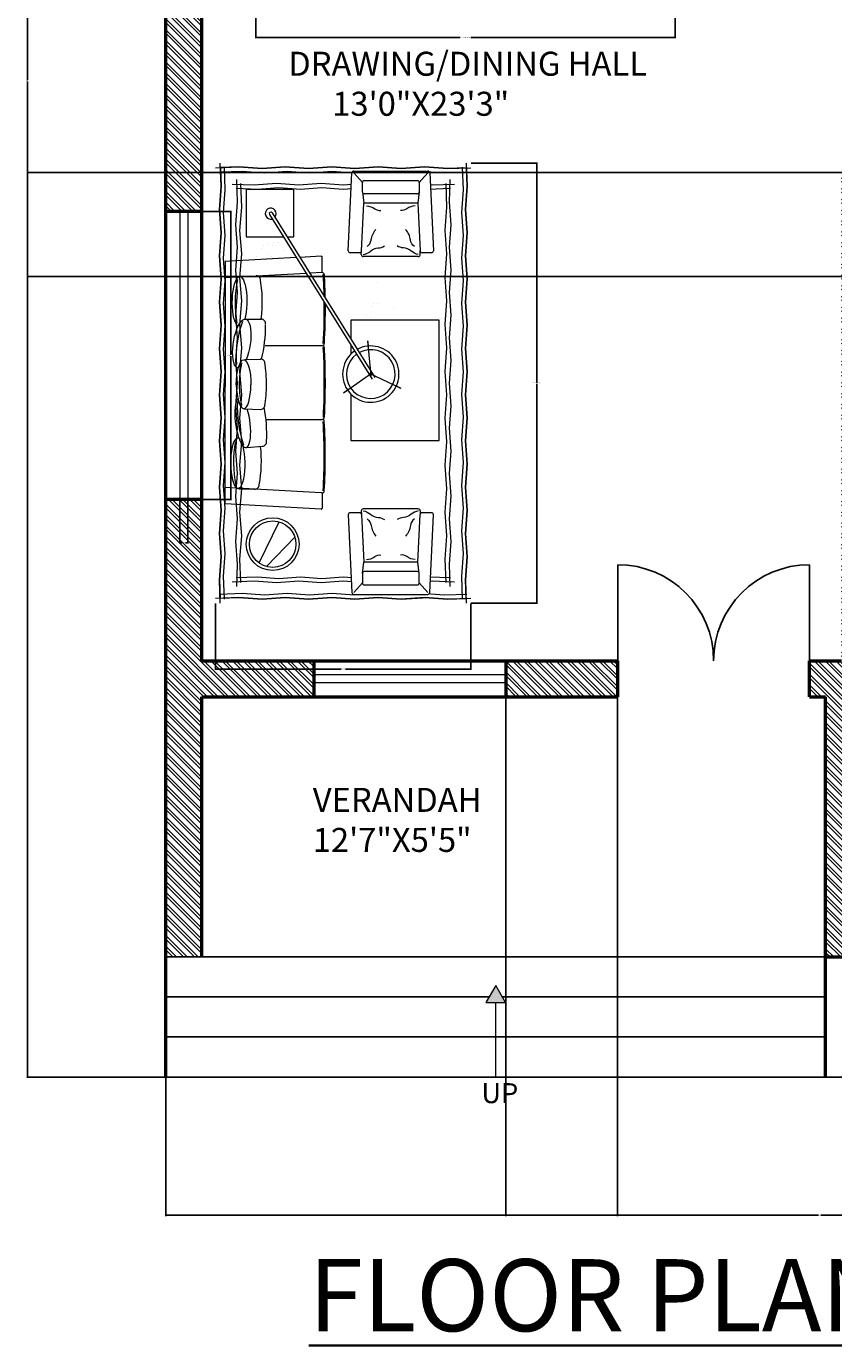
# Model space of a CAD drawing. Units: inches. Extents: x 10696 to 11614, y 5787 to 6498.
# Tile 1 of 9: x 10696 to 10898, y 5790 to 6120. Entities that reach past the tile are written whole.
import ezdxf

# ---------------------------------------------------------------- set-up
doc = ezdxf.new("R2010")
doc.units = ezdxf.units.IN
doc.set_wipeout_variables(frame=1)
for name, color, linetype, lineweight in [('A-ANNO-DIMS', 2, 'Continuous', 18), ('A-ANNO-SYMB', 2, 'Continuous', 18), ('A-ANNO-TITL', 7, 'Continuous', 35), ('A-AREA-IDEN', 7, 'Continuous', 25), ('A-DOOR', 3, 'Continuous', 25), ('A-FLOR', 7, 'Continuous', 25), ('A-FLOR-STRS', 7, 'Continuous', 25), ('A-FURN', 8, 'Continuous', 18), ('A-GLAZ', 4, 'Continuous', 20), ('A-WALL', 7, 'Continuous', 50), ('A-WALL-PATT', 252, 'Continuous', 13)]:
    doc.layers.add(name, color=color, linetype=linetype, lineweight=lineweight)
doc.styles.get("Standard").update_dxf_attribs({"font": 'arial.ttf'})
doc.dimstyles.get("Standard").update_dxf_attribs({"dimtxt": 0.18, "dimasz": 0.18, "dimexe": 0.18, "dimexo": 0.0625, "dimgap": 0.09, "dimtad": 0, "dimtih": 1, "dimtoh": 1, "dimdec": 4, "dimzin": 0, "dimdsep": 46, "dimtxsty": 'Standard', "dimcen": 0.09, "dimadec": 0, "dimazin": 0, "dimtfac": 1, "dimtdec": 4, "dimtofl": 0, "dimtmove": 0, "dimatfit": 3, "dimfxl": 1, "dimtolj": 1, "dimtzin": 0, "dimarcsym": 0})

# ---------------------------------------------------------------- blocks, each defined once
blk = doc.blocks.new('A$C7590614E')
for p, q in [((220, 4135), (46, 4129)), ((46, 4129), (52, 3952)), ((46, 4129), (46, 4129)), ((440, 4119), (220, 4135)), ((660, 4135), (440, 4119)), ((881, 4119), (660, 4135)), ((1101, 4135), (881, 4119)), ((1321, 4119), (1101, 4135)), ((1541, 4135), (1321, 4119)), ((1761, 4119), (1541, 4135)), ((1981, 4135), (1761, 4119)), ((2202, 4119), (1981, 4135)), ((2379, 4126), (2202, 4119)), ((2385, 3952), (2379, 4126)), ((52, 3952), (36, 3732)), ((2369, 3732), (2385, 3952)), ((36, 3732), (52, 3513)), ((2385, 3513), (2369, 3732)), ((52, 3513), (36, 3293)), ((496, 3597), (496, 3597)), ((596, 3620), (596, 3620)), ((2369, 3293), (2385, 3513)), ((454, 3393), (454, 3393)), ((492, 3396), (492, 3396)), ((536, 3390), (536, 3390)), ((553, 3416), (553, 3416)), ((592, 3420), (592, 3420)), ((36, 3293), (52, 3074)), ((765, 3275), (91, 3238)), ((392, 3284), (392, 3284)), ((426, 3262), (426, 3262)), ((436, 3366), (436, 3366)), ((492, 3308), (492, 3308)), ((526, 3286), (526, 3286)), ((641, 3347), (641, 3347)), ((741, 3371), (741, 3371)), ((1000, 3288), (799, 3277)), ((1011, 3134), (1011, 3278)), ((2385, 3074), (2369, 3293)), ((91, 3238), (91, 2051)), ((91, 3161), (91, 2051)), ((1010, 3133), (893, 3127)), ((52, 3074), (37, 2858)), ((859, 3125), (91, 3084)), ((236, 3098), (385, 3104)), ((374, 3100), (240, 3093)), ((332, 3098), (253, 3094)), ((1538, 3041), (1538, 3041)), ((2369, 2854), (2385, 3074)), ((37, 2858), (52, 2635)), ((1479, 2810), (1479, 2810)), ((1496, 2837), (1496, 2837)), ((1535, 2840), (1535, 2840)), ((1683, 2791), (1683, 2791)), ((2385, 2635), (2369, 2854)), ((52, 2635), (36, 2415)), ((276, 2693), (435, 2692)), ((1434, 2729), (1434, 2729)), ((1469, 2706), (1469, 2706)), ((2369, 2415), (2385, 2635)), ((36, 2415), (52, 2196)), ((469, 2441), (1012, 2441)), ((2385, 2196), (2369, 2415)), ((275, 2308), (424, 2314)), ((52, 2196), (36, 1976)), ((2369, 1976), (2385, 2196)), ((91, 941), (91, 2051)), ((91, 941), (91, 2051)), ((36, 1976), (52, 1756)), ((2385, 1756), (2369, 1976)), ((52, 1756), (36, 1537)), ((275, 1842), (424, 1836)), ((2369, 1537), (2385, 1756)), ((478, 1742), (1012, 1742)), ((36, 1537), (52, 1317)), ((2385, 1317), (2369, 1537)), ((296, 1474), (445, 1487)), ((52, 1317), (36, 1098)), ((2369, 1098), (2385, 1317)), ((36, 1098), (52, 878)), ((1001, 1045), (91, 1095)), ((221, 1085), (370, 1080)), ((1010, 1045), (1001, 1045)), ((1011, 1045), (1011, 901)), ((2385, 878), (2369, 1098)), ((52, 878), (36, 659)), ((1001, 891), (91, 941)), ((2369, 659), (2385, 878)), ((36, 659), (52, 439)), ((2385, 439), (2369, 659)), ((52, 439), (36, 220)), ((2369, 220), (2385, 439)), ((36, 220), (43, 46)), ((2376, 43), (2369, 220)), ((43, 46), (220, 52)), ((220, 52), (440, 36)), ((440, 36), (660, 52)), ((660, 52), (881, 36)), ((881, 36), (1101, 52)), ((1101, 52), (1321, 36)), ((1321, 36), (1541, 52)), ((1541, 52), (1761, 36)), ((1761, 36), (1966, 51)), ((1966, 51), (1981, 52)), ((1981, 52), (2202, 36)), ((2202, 36), (2376, 43))]:
    blk.add_line(p, q)
at = {"linetype": 'ByBlock'}
for p, q in [((1474, 2154, 0), (1445, 2485, 0)), ((1474, 2154, 0), (1445, 2485, 0)), ((1450, 2427, 0), (1446, 2481, 0)), ((1487, 2182, 0), (1213, 1991, 0)), ((1487, 2182, 0), (1213, 1991, 0)), ((1456, 2179, 0), (1757, 2037, 0)), ((1456, 2179, 0), (1757, 2037, 0)), ((1261, 2025, 0), (1217, 1994, 0)), ((1705, 2062, 0), (1754, 2039, 0)), ((412, 381), (604, 770)), ((751, 626), (481, 348))]:
    blk.add_line(p, q, dxfattribs=at)
at = {"linetype": 'ByBlock', "flags": 128}
for points in [[(0, 4127), (220, 4135), (440, 4119), (660, 4135), (881, 4119), (1101, 4135), (1321, 4119), (1541, 4135), (1761, 4119), (1981, 4135), (2202, 4119), (2422, 4127)], [(44, 0), (36, 220), (52, 439), (36, 659), (52, 878), (36, 1098), (52, 1317), (36, 1537), (52, 1756), (36, 1976), (52, 2196), (36, 2415), (52, 2635), (36, 2854), (52, 3074), (36, 3293), (52, 3513), (36, 3732), (52, 3952), (44, 4172)], [(83, 39), (75, 254), (91, 470), (75, 685), (91, 901), (75, 1116), (91, 1332), (75, 1547), (91, 1763), (75, 1978), (91, 2194), (75, 2409), (91, 2624), (75, 2840), (91, 3055), (75, 3271), (91, 3486), (75, 3702), (91, 3917), (83, 4133)], [(2339, 4133), (2347, 3917), (2331, 3702), (2347, 3486), (2331, 3271), (2347, 3055), (2331, 2840), (2347, 2624), (2331, 2409), (2347, 2194), (2331, 1978), (2347, 1763), (2331, 1547), (2347, 1332), (2331, 1116), (2347, 901), (2331, 685), (2347, 470), (2331, 254), (2339, 39)], [(2377, 4172), (2385, 3952), (2369, 3732), (2385, 3513), (2369, 3293), (2385, 3074), (2369, 2854), (2385, 2635), (2369, 2415), (2385, 2196), (2369, 1976), (2385, 1756), (2369, 1537), (2385, 1317), (2369, 1098), (2385, 878), (2369, 659), (2385, 439), (2369, 220), (2377, 0)], [(39, 4088), (252, 4096), (465, 4080), (678, 4096), (891, 4080), (1104, 4096), (1317, 4080), (1531, 4096), (1744, 4080), (1957, 4096), (2170, 4080), (2383, 4088)], [(200, 156), (208, 370), (192, 584), (208, 799), (192, 1013), (208, 1228), (192, 1442), (208, 1657), (192, 1871), (208, 2086), (192, 2300), (208, 2515), (192, 2729), (208, 2944), (192, 3158), (208, 3373), (192, 3587), (208, 3802), (200, 4016)], [(2222, 4016), (2214, 3802), (2230, 3587), (2214, 3373), (2230, 3158), (2214, 2944), (2230, 2729), (2214, 2515), (2230, 2300), (2214, 2086), (2230, 1871), (2214, 1657), (2230, 1442), (2214, 1228), (2230, 1013), (2214, 799), (2230, 584), (2214, 370), (2222, 156)], [(156, 3972), (367, 3964), (578, 3980), (789, 3964), (1000, 3980), (1211, 3964), (1422, 3980), (1633, 3964), (1844, 3980), (2055, 3964), (2266, 3972)], [(194, 3933), (398, 3925), (601, 3941), (804, 3925), (1008, 3941), (1211, 3925), (1414, 3941), (1617, 3925), (1821, 3941), (2024, 3925), (2227, 3933)], [(239, 194), (231, 417), (247, 639), (231, 862), (247, 1084), (231, 1307), (247, 1529), (231, 1752), (247, 1975), (231, 2197), (247, 2420), (231, 2642), (247, 2865), (231, 3087), (247, 3310), (231, 3532), (247, 3755), (239, 3977)], [(2183, 3977), (2191, 3755), (2175, 3532), (2191, 3310), (2175, 3087), (2191, 2865), (2175, 2642), (2191, 2420), (2175, 2197), (2191, 1975), (2175, 1752), (2191, 1529), (2175, 1307), (2191, 1084), (2175, 862), (2191, 639), (2175, 417), (2183, 194)], [(2266, 200), (2055, 208), (1844, 192), (1633, 208), (1422, 192), (1211, 208), (1000, 192), (789, 208), (578, 192), (367, 208), (156, 200)], [(2227, 239), (2024, 247), (1821, 231), (1617, 247), (1414, 231), (1211, 247), (1008, 231), (804, 247), (601, 231), (398, 247), (194, 239)], [(2422, 44), (2202, 36), (1981, 52), (1761, 36), (1541, 52), (1321, 36), (1101, 52), (881, 36), (660, 52), (440, 36), (220, 52), (0, 44)], [(2383, 83), (2170, 75), (1957, 91), (1744, 75), (1531, 91), (1317, 75), (1104, 91), (891, 75), (678, 91), (465, 75), (252, 91), (39, 83)]]:
    blk.add_lwpolyline(points, dxfattribs=at)
at = {"linetype": 'ByBlock'}
blk.add_lwpolyline([(678, 3471), (741, 3471), (741, 3921), (291, 3921), (291, 3471), (643, 3471)], dxfattribs=at)
for points in [[(1282, 1984), (1282, 1541), (2122, 1541), (2122, 2681), (1282, 2681), (1282, 2504)], [(1282, 2447), (1282, 2359)]]:
    blk.add_lwpolyline(points)
at = {"linetype": 'ByBlock', "const_width": 10, "elevation": 0}
for points in [[(1450, 2427), (1446, 2481)], [(1261, 2025), (1217, 1994)], [(1705, 2062), (1754, 2039)]]:
    blk.add_lwpolyline(points, dxfattribs=at)
at = {"linetype": 'ByBlock'}
for radius in [250, 220]:
    blk.add_circle((541, 559), radius, dxfattribs=at)
for radius, start, end in [(52.4, 318.5939, 285.3184), (15, 31.9562, 211.9562)]:
    blk.add_arc((523, 3692), radius, start, end, dxfattribs=at)
for centre, radius, start, end in [((1001, 3278), 10, 0, 93.0128), ((1011, 3113), 20, 3.7459, 93.0128), ((1254, 2846), 1070, 168.034, 190.3551), ((-385, 2845), 798, 18.6145, 18.6419), ((387, 3061), 42.5, 33.8407, 92.0223), ((-822, 2855), 1265, 352.6106, 10.4711), ((-4595, 2788), 5626, 1.223, 3.3226), ((-4595, 2788), 5636, 1.0525, 3.3226), ((-4595, 2788), 5626, 356.669, 0.6303), ((-4595, 2788), 5636, 356.669, 0.4637), ((1265, 2321), 1070, 160.9121, 183.2331), ((431, 2650), 42.5, 352.6116, 84.9003), ((-796, 2619), 1269, 346.0345, 0.8134), ((1011, 2421), 20, 3.742, 91.3972), ((1011, 2461), 20, 271.3972, 356.2445), ((-2252, 2185), 3282, 359.485, 4.1508), ((-2252, 2185), 3292, 359.485, 4.1508), ((1293, 2055), 1070, 168.034, 179.2769), ((425, 2271), 42.5, 16.3929, 92.0223), ((-783, 2085), 1265, 359.2714, 9.0059), ((425, 2271), 42.5, 359.7336, 1.1068), ((-4089, 2069), 5120, 356.563, 0.9635), ((-4089, 2069), 5130, 356.563, 0.9635), ((1293, 2094), 1070, 181.3636, 191.966), ((-783, 2065), 1265, 350.9941, 0.1868), ((1275, 1851), 1070, 176.7669, 199.0879), ((425, 1879), 42.5, 358.8932, 0.2664), ((425, 1879), 42.5, 267.9777, 343.6071), ((-780, 1606), 1265, 356.7804, 11.4363), ((1011, 1762), 20, 268.6028, 356.258), ((1011, 1722), 20, 3.7555, 88.6028), ((-4697, 1393), 5727, 356.706, 3.3024), ((-4697, 1393), 5737, 356.706, 3.3024), ((1239, 1338), 1070, 169.6449, 191.966), ((441, 1530), 42.5, 275.0997, 7.3884), ((-831, 1350), 1265, 349.6584, 6.1656), ((-400, 1339), 798, 341.3581, 341.3855), ((371, 1122), 42.5, 267.9777, 0.2664), ((1011, 1065), 20, 266.9872, 356.2541), ((1001, 901), 10, 266.9872, 0)]:
    blk.add_arc(centre, radius, start, end)
at = {"extrusion": (0, 0, -1)}
for centre, major_axis, ratio, start_param, end_param in [((227, 2858), (2, 239), 0.289653, 3.343252, 8.61472), ((248, 2460), (35, 232), 0.342983, 3.115548, 8.511087), ((265, 2068), (2, 239), 0.289653, -1.56819, 1.564113)]:
    blk.add_ellipse(centre, major_axis=major_axis, ratio=ratio, start_param=start_param, end_param=end_param, dxfattribs=at)
at = {"linetype": 'ByBlock', "extrusion": (3.38184e-09, 2.26187e-09, 1)}
for major_axis, start_param, end_param in [((-219, -153, 0), 4.720612, 10.891434), ((-190, -132, 0), 4.729628, 10.883141)]:
    blk.add_ellipse((1472, 2171), major_axis=major_axis, ratio=1, start_param=start_param, end_param=end_param, dxfattribs=at)
for centre, major_axis, start_param, end_param in [((265, 2082), (-2, 239), 1.623473, 4.655635), ((257, 1711), (-31, 237), 0.253375, 5.250818), ((211, 1326), (-2, 239), -0.16583, 5.452765)]:
    blk.add_ellipse(centre, major_axis=major_axis, ratio=0.289653, start_param=start_param, end_param=end_param)
for points in [[(1941, 3334), (1941, 3305), (1940, 3297), (1936, 3292), (1929, 3287), (1929, 3287), (1919, 3286), (1838, 3286), (1732, 3286), (1653, 3286), (1475, 3286), (1400, 3286), (1392, 3288), (1387, 3292), (1383, 3298), (1382, 3305), (1382, 3311), (1383, 3317), (1383, 3329), (1383, 3336), (1378, 3327), (1372, 3323), (1366, 3322), (1359, 3322), (1271, 3323), (1263, 3328), (1263, 3328), (1259, 3334), (1258, 3341), (1258, 3341), (1292, 4079), (1294, 4086), (1297, 4091), (1297, 4091), (1310, 4096), (1316, 4096), (1326, 4096), (1336, 4096), (2002, 4096), (2014, 4096), (2026, 4091), (2032, 4079), (2032, 4070), (2066, 3341), (2061, 3328), (2061, 3328), (2048, 3322), (2028, 3322), (1992, 3322), (1958, 3322), (1951, 3324), (1945, 3327), (1944, 3329)], [(1941, 845), (1941, 874), (1940, 882), (1936, 887), (1929, 892), (1929, 892), (1919, 893), (1838, 893), (1732, 893), (1653, 893), (1475, 893), (1400, 893), (1392, 891), (1387, 887), (1383, 881), (1382, 874), (1382, 868), (1383, 862), (1383, 850), (1383, 843), (1378, 852), (1372, 856), (1366, 857), (1359, 857), (1271, 856), (1263, 851), (1263, 851), (1259, 845), (1258, 838), (1258, 838), (1292, 100), (1294, 93), (1297, 88), (1297, 88), (1310, 83), (1316, 83), (1326, 83), (1336, 83), (2002, 83), (2014, 83), (2026, 88), (2032, 100), (2032, 109), (2066, 838), (2061, 851), (2061, 851), (2048, 857), (2028, 857), (1992, 857), (1958, 857), (1951, 855), (1945, 852), (1944, 850)]]:
    blk.add_wipeout(points).translate(0, 0, 0)
at = {"linetype": 'ByBlock'}
for p, q in [((1258, 3341, 0), (1292, 4079, 0)), ((1310, 4096, 0), (2014, 4096, 0)), ((1310, 4078, 0), (1392, 3988, 0)), ((1310, 4078, 0), (1392, 3988, 0)), ((1410, 4006, 0), (1914, 4006, 0)), ((1410, 4006, 0), (1914, 4006, 0)), ((2014, 4078, 0), (1932, 3988, 0)), ((2014, 4078, 0), (1932, 3988, 0)), ((2032, 4079, 0), (2066, 3341, 0)), ((1392, 3898, 0), (1392, 3988, 0)), ((1392, 3898, 0), (1392, 3988, 0)), ((1392, 3898, 0), (1405, 3792, 0)), ((1392, 3898, 0), (1405, 3792, 0)), ((1914, 3880, 0), (1410, 3880, 0)), ((1914, 3880, 0), (1410, 3880, 0)), ((1932, 3898, 0), (1919, 3792, 0)), ((1932, 3898, 0), (1919, 3792, 0)), ((1932, 3988, 0), (1932, 3898, 0)), ((1932, 3988, 0), (1932, 3898, 0)), ((1384, 3339, 0), (1405, 3792, 0)), ((1384, 3339, 0), (1405, 3792, 0)), ((1919, 3792, 0), (1405, 3792, 0)), ((1919, 3792, 0), (1405, 3792, 0)), ((1919, 3792, 0), (1940, 3339, 0)), ((1919, 3792, 0), (1940, 3339, 0)), ((510, 3684), (1484, 2123)), ((536, 3700), (1510, 2138)), ((1366, 3322, 0), (1276, 3322, 0)), ((1382, 3305, 0), (1384, 3339, 0)), ((1923, 3286, 0), (1400, 3286, 0)), ((1941, 3305, 0), (1940, 3339, 0)), ((2048, 3322, 0), (1958, 3322, 0)), ((1923, 893, 0), (1400, 893, 0)), ((1258, 838, 0), (1292, 100, 0)), ((1366, 857, 0), (1276, 857, 0)), ((1382, 874, 0), (1384, 840, 0)), ((1384, 840, 0), (1405, 387, 0)), ((1384, 840, 0), (1405, 387, 0)), ((1919, 387, 0), (1940, 840, 0)), ((1919, 387, 0), (1940, 840, 0)), ((1941, 874, 0), (1940, 840, 0)), ((2048, 857, 0), (1958, 857, 0)), ((2032, 100, 0), (2066, 838, 0)), ((1392, 281, 0), (1405, 387, 0)), ((1392, 281, 0), (1405, 387, 0)), ((1919, 387, 0), (1405, 387, 0)), ((1919, 387, 0), (1405, 387, 0)), ((1932, 281, 0), (1919, 387, 0)), ((1932, 281, 0), (1919, 387, 0)), ((1392, 281, 0), (1392, 191, 0)), ((1392, 281, 0), (1392, 191, 0)), ((1914, 299, 0), (1410, 299, 0)), ((1914, 299, 0), (1410, 299, 0)), ((1932, 191, 0), (1932, 281, 0)), ((1932, 191, 0), (1932, 281, 0)), ((1310, 101, 0), (1392, 191, 0)), ((1310, 101, 0), (1392, 191, 0)), ((1410, 173, 0), (1914, 173, 0)), ((1410, 173, 0), (1914, 173, 0)), ((2014, 101, 0), (1932, 191, 0)), ((2014, 101, 0), (1932, 191, 0)), ((1310, 83, 0), (2014, 83, 0))]:
    blk.add_line(p, q, dxfattribs=at)
at = {"linetype": 'ByBlock', "elevation": 0}
for points in [[(1430, 3765, -0.157856), (1510, 3738, 0.195258), (1568, 3723, 0.506042)], [(1430, 3765, -0.157856), (1510, 3738, 0.195258), (1568, 3723, 0.506042)], [(1894, 3765, 0.157856), (1813, 3738, -0.195258), (1755, 3723, -0.506042)], [(1894, 3765, 0.157856), (1813, 3738, -0.195258), (1755, 3723, -0.506042)], [(1437, 3380, 0.215808), (1475, 3442, -0.158378), (1521, 3543, -0.75133)], [(1437, 3380, 0.215808), (1475, 3442, -0.158378), (1521, 3543, -0.75133)], [(1886, 3380, -0.215808), (1849, 3442, 0.158378), (1802, 3543, 0.75133)], [(1886, 3380, -0.215808), (1849, 3442, 0.158378), (1802, 3543, 0.75133)], [(1400, 3304, 0.13045), (1468, 3337, -0.166434), (1542, 3367, 0.138962), (1601, 3387, -0.132288)], [(1400, 3304, 0.13045), (1468, 3337, -0.166434), (1542, 3367, 0.138962), (1601, 3387, -0.132288)], [(1923, 3304, -0.13045), (1856, 3337, 0.166434), (1781, 3367, -0.138962), (1723, 3387, 0.132288)], [(1923, 3304, -0.13045), (1856, 3337, 0.166434), (1781, 3367, -0.138962), (1723, 3387, 0.132288)], [(1400, 875, -0.13045), (1468, 842, 0.166434), (1542, 812, -0.138962), (1601, 792, 0.132288)], [(1400, 875, -0.13045), (1468, 842, 0.166434), (1542, 812, -0.138962), (1601, 792, 0.132288)], [(1437, 799, -0.215808), (1475, 737, 0.158378), (1521, 636, 0.75133)], [(1437, 799, -0.215808), (1475, 737, 0.158378), (1521, 636, 0.75133)], [(1923, 875, 0.13045), (1856, 842, -0.166434), (1781, 812, 0.138962), (1723, 792, -0.132288)], [(1923, 875, 0.13045), (1856, 842, -0.166434), (1781, 812, 0.138962), (1723, 792, -0.132288)], [(1886, 799, 0.215808), (1849, 737, -0.158378), (1802, 636, -0.75133)], [(1886, 799, 0.215808), (1849, 737, -0.158378), (1802, 636, -0.75133)], [(1430, 414, 0.157856), (1510, 441, -0.195258), (1568, 456, -0.506042)], [(1430, 414, 0.157856), (1510, 441, -0.195258), (1568, 456, -0.506042)], [(1894, 414, -0.157856), (1813, 441, 0.195258), (1755, 456, 0.506042)], [(1894, 414, -0.157856), (1813, 441, 0.195258), (1755, 456, 0.506042)]]:
    blk.add_lwpolyline(points, format="xyb", dxfattribs=at)
at = {"linetype": 'ByBlock'}
for centre, start, end in [((1310, 4078, 0), 90, 177.337), ((1410, 3988, 0), 90, 180), ((1410, 3988, 0), 90, 180), ((1914, 3988, 0), 0, 90), ((1914, 3988, 0), 0, 90), ((2014, 4078, 0), 2.663, 90), ((1410, 3898, 0), 180, 270), ((1410, 3898, 0), 180, 270), ((1914, 3898, 0), 270, 0), ((1914, 3898, 0), 270, 0), ((1276, 3340, 0), 177.337, 270), ((1366, 3340, 0), 270, 357.337), ((1400, 3304, 0), 177.337, 270), ((1923, 3304, 0), 270, 2.663), ((1958, 3340, 0), 182.663, 270), ((2048, 3340, 0), 270, 2.663), ((1400, 875, 0), 90, 182.663), ((1923, 875, 0), 357.337, 90), ((1276, 839, 0), 90, 182.663), ((1366, 839, 0), 2.663, 90), ((1958, 839, 0), 90, 177.337), ((2048, 839, 0), 357.337, 90), ((1410, 281, 0), 90, 180), ((1410, 281, 0), 90, 180), ((1914, 281, 0), 360, 90), ((1914, 281, 0), 360, 90), ((1410, 191, 0), 180, 270), ((1410, 191, 0), 180, 270), ((1914, 191, 0), 270, 360), ((1914, 191, 0), 270, 360), ((1310, 101, 0), 182.663, 270), ((2014, 101, 0), 270, 357.337)]:
    blk.add_arc(centre, 18, start, end, dxfattribs=at)
blk = doc.blocks.new('DOOR-PAIR-48')
for p, q in [((0, 0), (0, 24)), ((48, 0), (48, 24))]:
    blk.add_line(p, q)
for centre, start, end in [((0, 0), 0, 90), ((48, 0), 90, 180)]:
    blk.add_arc(centre, 24, start, end)
blk = doc.blocks.new('WIN-GLAZ-48')
for p, q in [((0, 48), (0, 0)), ((2, 48), (2, 0))]:
    blk.add_line(p, q)
blk = doc.blocks.new('WIN-GLAZ-72')
for p, q in [((0, 72), (0, 0)), ((2, 72), (2, 0))]:
    blk.add_line(p, q)
blk = doc.blocks.new('*D32')
at = {"layer": 'A-ANNO-DIMS', "color": 0, "lineweight": -2, "transparency": 16777216}
for p, q in [((10736.48, 6073.33), (10747.39, 6073.33)), ((10747.21, 6073.15), (10747.21, 6037.52)), ((10747.21, 6001.51), (10747.21, 6037.15)), ((10736.48, 6001.33), (10747.39, 6001.33))]:
    blk.add_line(p, q, dxfattribs=at)
at = {"layer": 'A-ANNO-DIMS', "color": 0, "transparency": 16777216}
for points in [[(10747.18, 6073.15), (10747.24, 6073.15), (10747.21, 6073.33)], [(10747.18, 6001.51), (10747.24, 6001.51), (10747.21, 6001.33)]]:
    blk.add_solid(points, dxfattribs=at)
at = {"layer": 'Defpoints', "color": 0, "transparency": 16777216}
for p in [(10736.41, 6073.33), (10747.21, 6073.33), (10736.41, 6001.33)]:
    blk.add_point(p, dxfattribs=at)
at = {"layer": 'A-ANNO-DIMS', "color": 0, "transparency": 16777216, "insert": (10747.21, 6037.33), "char_height": 0.18, "attachment_point": 5}
blk.add_mtext('\\A1;WINDOW 72 TYP.', dxfattribs=at)
blk = doc.blocks.new('*D33')
at = {"layer": 'A-ANNO-DIMS', "color": 0, "lineweight": -2, "transparency": 16777216}
for p, q in [((10734.41, 6001.27), (10734.41, 5990.35)), ((10736.41, 6001.27), (10736.41, 5990.35)), ((10734.59, 5990.53), (10734.95, 5990.53)), ((10736.23, 5990.53), (10735.87, 5990.53))]:
    blk.add_line(p, q, dxfattribs=at)
at = {"layer": 'A-ANNO-DIMS', "color": 0, "transparency": 16777216}
for points in [[(10734.59, 5990.56), (10734.59, 5990.5), (10734.41, 5990.53)], [(10736.23, 5990.56), (10736.23, 5990.5), (10736.41, 5990.53)]]:
    blk.add_solid(points, dxfattribs=at)
at = {"layer": 'Defpoints', "color": 0, "transparency": 16777216}
for p in [(10734.41, 6001.33), (10736.41, 6001.33), (10736.41, 5990.53)]:
    blk.add_point(p, dxfattribs=at)
at = {"layer": 'A-ANNO-DIMS', "color": 0, "transparency": 16777216, "insert": (10735.41, 5990.53), "char_height": 0.18, "attachment_point": 5}
blk.add_mtext('\\A1;2 TYP.', dxfattribs=at)
blk = doc.blocks.new('*D36')
at = {"layer": 'A-ANNO-DIMS', "color": 0, "lineweight": -2, "transparency": 16777216}
for p, q in [((10753.44, 6132.46), (10753.44, 6116.62)), ((10858.3, 6132.46), (10858.3, 6116.62)), ((10753.62, 6116.8), (10804.52, 6116.8)), ((10858.12, 6116.8), (10807.22, 6116.8))]:
    blk.add_line(p, q, dxfattribs=at)
at = {"layer": 'A-ANNO-DIMS', "color": 0, "transparency": 16777216}
for points in [[(10753.62, 6116.83), (10753.62, 6116.77), (10753.44, 6116.8)], [(10858.12, 6116.83), (10858.12, 6116.77), (10858.3, 6116.8)]]:
    blk.add_solid(points, dxfattribs=at)
at = {"layer": 'Defpoints', "color": 0, "transparency": 16777216}
for p in [(10753.44, 6132.52), (10858.3, 6132.52), (10858.3, 6116.8)]:
    blk.add_point(p, dxfattribs=at)
at = {"layer": 'A-ANNO-DIMS', "color": 0, "transparency": 16777216, "insert": (10805.87, 6116.8), "char_height": 0.18, "attachment_point": 5}
blk.add_mtext('\\A1;DINING SET 105 TYP.', dxfattribs=at)
blk = doc.blocks.new('*D38')
at = {"layer": 'A-ANNO-DIMS', "color": 0, "lineweight": -2, "transparency": 16777216}
for p, q in [((10807.27, 6085.41), (10823.88, 6085.41)), ((10823.7, 6085.23), (10823.7, 6030.63)), ((10823.7, 5975.65), (10823.7, 6030.26)), ((10807.27, 5975.47), (10823.88, 5975.47))]:
    blk.add_line(p, q, dxfattribs=at)
at = {"layer": 'A-ANNO-DIMS', "color": 0, "transparency": 16777216}
for points in [[(10823.67, 6085.23), (10823.73, 6085.23), (10823.7, 6085.41)], [(10823.67, 5975.65), (10823.73, 5975.65), (10823.7, 5975.47)]]:
    blk.add_solid(points, dxfattribs=at)
at = {"layer": 'Defpoints', "color": 0, "transparency": 16777216}
for p in [(10807.21, 6085.41), (10823.7, 6085.41), (10807.21, 5975.47)]:
    blk.add_point(p, dxfattribs=at)
at = {"layer": 'A-ANNO-DIMS', "color": 0, "transparency": 16777216, "insert": (10823.7, 6030.44), "char_height": 0.18, "attachment_point": 5}
blk.add_mtext('\\A1;SOFA SET 110 TYP.', dxfattribs=at)
blk = doc.blocks.new('*D39')
at = {"layer": 'A-ANNO-DIMS', "color": 0, "lineweight": -2, "transparency": 16777216}
for p, q in [((10743.39, 5975.41), (10743.39, 5958.8)), ((10807.21, 5975.41), (10807.21, 5958.8)), ((10743.57, 5958.98), (10774.77, 5958.98)), ((10807.03, 5958.98), (10775.83, 5958.98))]:
    blk.add_line(p, q, dxfattribs=at)
at = {"layer": 'A-ANNO-DIMS', "color": 0, "transparency": 16777216}
for points in [[(10743.57, 5959.01), (10743.57, 5958.95), (10743.39, 5958.98)], [(10807.03, 5959.01), (10807.03, 5958.95), (10807.21, 5958.98)]]:
    blk.add_solid(points, dxfattribs=at)
at = {"layer": 'Defpoints', "color": 0, "transparency": 16777216}
for p in [(10743.39, 5975.47), (10807.21, 5975.47), (10807.21, 5958.98)]:
    blk.add_point(p, dxfattribs=at)
at = {"layer": 'A-ANNO-DIMS', "color": 0, "transparency": 16777216, "insert": (10775.3, 5958.98), "char_height": 0.18, "attachment_point": 5}
blk.add_mtext('\\A1;64 TYP.', dxfattribs=at)
blk = doc.blocks.new('*D70')
at = {"layer": 'A-ANNO-DIMS', "color": 0, "lineweight": -2, "transparency": 16777216}
for p, q in [((10730.91, 5887.01), (10730.91, 5822.34)), ((11057.91, 5887.01), (11057.91, 5822.34)), ((10731.09, 5822.52), (10894.12, 5822.52)), ((11057.73, 5822.52), (10894.7, 5822.52))]:
    blk.add_line(p, q, dxfattribs=at)
at = {"layer": 'A-ANNO-DIMS', "color": 0, "transparency": 16777216}
for points in [[(10731.09, 5822.55), (10731.09, 5822.49), (10730.91, 5822.52)], [(11057.73, 5822.55), (11057.73, 5822.49), (11057.91, 5822.52)]]:
    blk.add_solid(points, dxfattribs=at)
at = {"layer": 'Defpoints', "color": 0, "transparency": 16777216}
for p in [(10730.91, 5887.07), (11057.91, 5887.07), (11057.91, 5822.52)]:
    blk.add_point(p, dxfattribs=at)
at = {"layer": 'A-ANNO-DIMS', "color": 0, "transparency": 16777216, "insert": (10894.41, 5822.52), "char_height": 0.18, "attachment_point": 5}
blk.add_mtext('\\A1;327', dxfattribs=at)
blk = doc.blocks.new('*D71')
at = {"layer": 'A-ANNO-DIMS', "color": 0, "lineweight": -2, "transparency": 16777216}
for p, q in [((10816.99, 6354.91), (10696.18, 6354.91)), ((10696.36, 6354.73), (10696.36, 6106.17)), ((10696.36, 5857.25), (10696.36, 6105.81)), ((10730.85, 5857.07), (10696.18, 5857.07))]:
    blk.add_line(p, q, dxfattribs=at)
at = {"layer": 'A-ANNO-DIMS', "color": 0, "transparency": 16777216}
for points in [[(10696.33, 6354.73), (10696.39, 6354.73), (10696.36, 6354.91)], [(10696.33, 5857.25), (10696.39, 5857.25), (10696.36, 5857.07)]]:
    blk.add_solid(points, dxfattribs=at)
at = {"layer": 'Defpoints', "color": 0, "transparency": 16777216}
for p in [(10696.36, 6354.91), (10817.05, 6354.91), (10730.91, 5857.07)]:
    blk.add_point(p, dxfattribs=at)
at = {"layer": 'A-ANNO-DIMS', "color": 0, "transparency": 16777216, "insert": (10696.36, 6105.99), "char_height": 0.18, "attachment_point": 5}
blk.add_mtext('\\A1;497.8', dxfattribs=at)
blk = doc.blocks.new('*D74')
at = {"layer": 'A-ANNO-DIMS', "color": 0, "lineweight": -2, "transparency": 16777216}
for p, q in [((10895.98, 5887.07), (11092.64, 5887.07)), ((11092.46, 5886.89), (11092.46, 5872.25)), ((11092.46, 5857.25), (11092.46, 5871.89)), ((10895.98, 5857.07), (11092.64, 5857.07))]:
    blk.add_line(p, q, dxfattribs=at)
at = {"layer": 'A-ANNO-DIMS', "color": 0, "transparency": 16777216}
for points in [[(11092.43, 5886.89), (11092.49, 5886.89), (11092.46, 5887.07)], [(11092.43, 5857.25), (11092.49, 5857.25), (11092.46, 5857.07)]]:
    blk.add_solid(points, dxfattribs=at)
at = {"layer": 'Defpoints', "color": 0, "transparency": 16777216}
for p in [(10895.91, 5887.07), (11092.46, 5887.07), (10895.91, 5857.07)]:
    blk.add_point(p, dxfattribs=at)
at = {"layer": 'A-ANNO-DIMS', "color": 0, "transparency": 16777216, "insert": (11092.46, 5872.07), "char_height": 0.18, "attachment_point": 5}
blk.add_mtext('\\A1;30', dxfattribs=at)
blk = doc.blocks.new('*D96')
at = {"layer": 'A-ANNO-DIMS', "color": 0, "lineweight": -2, "transparency": 16777216}
for p, q in [((10815.91, 5952.01), (10815.91, 5822.34)), ((10843.91, 5952.01), (10843.91, 5822.34)), ((10816.09, 5822.52), (10829.69, 5822.52)), ((10843.73, 5822.52), (10830.13, 5822.52))]:
    blk.add_line(p, q, dxfattribs=at)
at = {"layer": 'A-ANNO-DIMS', "color": 0, "transparency": 16777216}
for points in [[(10816.09, 5822.55), (10816.09, 5822.49), (10815.91, 5822.52)], [(10843.73, 5822.55), (10843.73, 5822.49), (10843.91, 5822.52)]]:
    blk.add_solid(points, dxfattribs=at)
at = {"layer": 'Defpoints', "color": 0, "transparency": 16777216}
for p in [(10815.91, 5952.07), (10843.91, 5952.07), (10843.91, 5822.52)]:
    blk.add_point(p, dxfattribs=at)
at = {"layer": 'A-ANNO-DIMS', "color": 0, "transparency": 16777216, "insert": (10829.91, 5822.52), "char_height": 0.18, "attachment_point": 5}
blk.add_mtext('\\A1;28', dxfattribs=at)
blk = doc.blocks.new('*D98')
at = {"layer": 'A-ANNO-DIMS', "color": 0, "lineweight": -2, "transparency": 16777216}
for p, q in [((10952.85, 6083.07), (10696.18, 6083.07)), ((10696.36, 6082.89), (10696.36, 6070.25)), ((10696.36, 6057.25), (10696.36, 6069.89)), ((10952.85, 6057.07), (10696.18, 6057.07))]:
    blk.add_line(p, q, dxfattribs=at)
at = {"layer": 'A-ANNO-DIMS', "color": 0, "transparency": 16777216}
for points in [[(10696.33, 6082.89), (10696.39, 6082.89), (10696.36, 6083.07)], [(10696.33, 6057.25), (10696.39, 6057.25), (10696.36, 6057.07)]]:
    blk.add_solid(points, dxfattribs=at)
at = {"layer": 'Defpoints', "color": 0, "transparency": 16777216}
for p in [(10952.91, 6083.07), (10696.36, 6057.07), (10952.91, 6057.07)]:
    blk.add_point(p, dxfattribs=at)
at = {"layer": 'A-ANNO-DIMS', "color": 0, "transparency": 16777216, "insert": (10696.36, 6070.07), "char_height": 0.18, "attachment_point": 5}
blk.add_mtext('\\A1;26', dxfattribs=at)

msp = doc.modelspace()

# ---------------------------------------------------------------- hatches: boundary and pattern name
at = {"layer": 'A-ANNO-SYMB'}
h = msp.add_hatch(color=256, dxfattribs=at)
h.dxf.hatch_style = 1
h.paths.add_polyline_path([(10813.413, 5879.918), (10810.946, 5875.646), (10815.879, 5875.646)])
at = {"layer": 'A-WALL-PATT'}
h = msp.add_hatch(dxfattribs=at)
h.set_pattern_fill('ANSI32', color=256, scale=0.2, angle=90)
h.paths.add_polyline_path([(10767.913, 5961.07), (10739.913, 5961.07), (10739.913, 6001.333), (10730.913, 6001.333), (10730.913, 5887.07), (10739.913, 5887.07), (10739.913, 5952.07), (10767.913, 5952.07)])
h.paths.add_polyline_path([(10739.913, 6127.055), (10730.913, 6127.055), (10730.913, 6073.333), (10739.913, 6073.333)])
h.paths.add_polyline_path([(10739.913, 6267.869, -0.035413), (10740.694, 6278.876), (10731.784, 6280.146, 0.035413), (10730.913, 6267.869), (10730.913, 6199.055), (10739.913, 6199.055)])
h.paths.add_polyline_path([(10794.29, 6342.205), (10791.564, 6350.783, 0.1142038), (10757.817, 6330.777), (10764.034, 6324.269, -0.1142038)])
h.paths.add_polyline_path([(10844.262, 6350.783), (10841.536, 6342.205, -0.065871), (10860.057, 6333.503), (10864.919, 6341.077, 0.065871)])
h.paths.add_polyline_path([(10908.913, 6311.07), (10895.913, 6311.07), (10895.913, 6306.404, 0.0519949), (10886.285, 6321.667), (10879.212, 6316.101, -0.1682272), (10895.913, 6267.869), (10895.913, 6223.07), (10904.913, 6223.07), (10904.913, 6302.07), (10908.913, 6302.07)])
h.paths.add_polyline_path([(11057.913, 6311.07), (10944.913, 6311.07), (10944.913, 6302.07), (11048.913, 6302.07), (11048.913, 6273.514), (11057.913, 6273.514)])
h.paths.add_polyline_path([(11057.913, 6225.514), (11048.913, 6225.514), (11048.913, 6187.07), (10988.913, 6187.07), (10988.913, 6182.07), (11048.913, 6182.07), (11048.913, 6164.07), (11057.913, 6164.07)])
h.paths.add_polyline_path([(10952.913, 6187.07), (10895.913, 6187.07), (10895.913, 6182.07), (10948.913, 6182.07), (10948.913, 6113.07), (10952.913, 6113.07), (10952.913, 6117.07), (11048.913, 6117.07), (11048.913, 6099.07), (11057.913, 6099.07), (11057.913, 6140.07), (11048.913, 6140.07), (11048.913, 6122.07), (10952.913, 6122.07)])
h.paths.add_polyline_path([(11057.913, 6075.07), (11048.913, 6075.07), (11048.913, 6057.07), (10952.913, 6057.07), (10952.913, 6083.07), (10944.913, 6083.07), (10944.913, 6078.07), (10948.913, 6078.07), (10948.913, 6052.07), (11048.913, 6052.07), (11048.913, 6028.07), (11057.913, 6028.07)])
h.paths.add_polyline_path([(11057.913, 5992.07), (11048.913, 5992.07), (11048.913, 5896.07), (11000.913, 5896.07), (11000.913, 5887.07), (11057.913, 5887.07)])
h.paths.add_polyline_path([(10952.913, 5896.07), (10904.913, 5896.07), (10904.913, 6078.07), (10908.913, 6078.07), (10908.913, 6083.07), (10899.913, 6083.07), (10899.913, 5961.07), (10891.913, 5961.07), (10891.913, 5952.07), (10895.913, 5952.07), (10895.913, 5887.07), (10952.913, 5887.07)])
h.paths.add_polyline_path([(10843.913, 5961.07), (10815.913, 5961.07), (10815.913, 5952.07), (10843.913, 5952.07)])

# ---------------------------------------------------------------- linework, layer by layer
at = {"layer": 'A-ANNO-SYMB'}
msp.add_line((10813.413, 5857.07), (10813.413, 5875.646), dxfattribs=at)
msp.add_lwpolyline([(10813.413, 5879.918), (10810.946, 5875.646), (10815.879, 5875.646)], close=True, dxfattribs=at)
at = {"layer": 'A-FLOR'}
msp.add_line((10730.913, 5887.07), (10895.913, 5887.07), dxfattribs=at)
at = {"layer": 'A-FLOR-STRS'}
for p, q in [((10730.913, 5877.07), (10811.769, 5877.07)), ((10815.057, 5877.07), (10895.913, 5877.07)), ((10730.913, 5867.07), (10895.913, 5867.07)), ((10730.913, 5857.07), (10895.913, 5857.07))]:
    msp.add_line(p, q, dxfattribs=at)
at = {"layer": 'A-WALL'}
for p, q in [((10730.913, 5857.07), (10730.913, 6267.869)), ((10739.913, 5961.07), (10739.913, 6267.869)), ((10739.913, 6073.333), (10730.913, 6073.333)), ((10739.913, 6001.333), (10730.913, 6001.333)), ((10739.913, 5961.07), (10843.913, 5961.07)), ((10767.913, 5961.07), (10767.913, 5952.07)), ((10815.913, 5961.07), (10815.913, 5952.07)), ((10843.913, 5952.07), (10843.913, 5961.07)), ((10891.913, 5952.07), (10891.913, 5961.07)), ((10891.913, 5961.07), (10899.913, 5961.07)), ((10739.913, 5887.07), (10739.913, 5952.07)), ((10739.913, 5952.07), (10843.913, 5952.07)), ((10891.913, 5952.07), (10895.913, 5952.07)), ((10895.913, 5857.07), (10895.913, 5952.07)), ((10895.913, 5887.07), (11057.913, 5887.07))]:
    msp.add_line(p, q, dxfattribs=at)

# ---------------------------------------------------------------- block references
at = {"layer": 'A-DOOR'}
msp.add_blockref('DOOR-PAIR-48', (10843.913, 5961.07), dxfattribs=at)
at = {"layer": 'A-GLAZ'}
msp.add_blockref('WIN-GLAZ-72', (10734.413, 6001.333), dxfattribs=at)
at = {"layer": 'A-GLAZ', "rotation": 269.9999999999871}
msp.add_blockref('WIN-GLAZ-48', (10767.913, 5957.57), dxfattribs=at)

# ---------------------------------------------------------------- texts
at = {"layer": 'A-ANNO-SYMB', "insert": (10809.825, 5855.539), "char_height": 5, "attachment_point": 1}
msp.add_mtext_dynamic_manual_height_columns('UP', width=19.19633, gutter_width=12.5, heights=[0], dxfattribs=at)
at = {"layer": 'A-ANNO-TITL', "insert": (10766.66, 5811.558), "char_height": 18, "attachment_point": 1}
msp.add_mtext_dynamic_manual_height_columns('{\\LFLOOR PLAN}', width=251.84009, gutter_width=12.5, heights=[0], dxfattribs=at)
at = {"layer": 'A-AREA-IDEN', "char_height": 6, "attachment_point": 1}
for s, width, insert in [('DRAWING/DINING HALL\\P      13\'0"X23\'3"', 143.58411, (10761.538, 6113.237)), ('VERANDAH\\P12\'7"X5\'5"', 76.52537, (10767.675, 5929.31))]:
    msp.add_mtext_dynamic_manual_height_columns(s, width=width, gutter_width=12.5, heights=[0], dxfattribs=dict(at, insert=insert))

# ---------------------------------------------------------------- dimensions: what is measured, and where the dimension line sits
at = {"layer": 'A-ANNO-DIMS'}
for base, p1, p2, text, picture, middle in [((10858.298, 6116.795), (10753.443, 6132.524), (10858.298, 6132.524), 'DINING SET <> TYP.', '*D36', (10805.871, 6116.795)), ((10736.413, 5990.533), (10734.413, 6001.333), (10736.413, 6001.333), '<> TYP.', '*D33', (10735.413, 5990.533))]:
    dim = msp.add_linear_dim(base=base, p1=p1, p2=p2, text=text, dimstyle='Standard', override={"dimdec": 0, "dimlfac": 1, "dimrnd": 0, "dimzin": 0, "dimdsep": 46, "dimlunit": 2}, dxfattribs=at)
    dim.commit()
    dim.dimension.update_dxf_attribs({"geometry": picture, "text_midpoint": middle})
for base, p1, p2, picture, middle in [((10843.913, 5822.52), (10815.913, 5952.07), (10843.913, 5952.07), '*D96', (10829.913, 5822.52)), ((11057.913, 5822.52), (10730.913, 5887.07), (11057.913, 5887.07), '*D70', (10894.413, 5822.52))]:
    dim = msp.add_linear_dim(base=base, p1=p1, p2=p2, dimstyle='Standard', override={"dimdec": 0, "dimlfac": 1, "dimrnd": 0, "dimzin": 0, "dimdsep": 46, "dimlunit": 2}, dxfattribs=at)
    dim.commit()
    dim.dimension.update_dxf_attribs({"geometry": picture, "text_midpoint": middle})
dim = msp.add_linear_dim(base=(11092.463, 5887.07), p1=(10895.913, 5857.07), p2=(10895.913, 5887.07), angle=90, dimstyle='Standard', override={"dimdec": 0, "dimlfac": 1, "dimrnd": 0, "dimzin": 0, "dimdsep": 46, "dimlunit": 2}, dxfattribs=at)
dim.commit()
dim.dimension.update_dxf_attribs({"geometry": '*D74', "text_midpoint": (11092.463, 5872.07)})

# ---------------------------------------------------------------- next in the draw order: block references
at = {"layer": 'A-FURN', "xscale": 0.0263548390649643, "yscale": 0.0263548390649643, "zscale": 0.0263548390649643}
msp.add_blockref('A$C7590614E', (10743.387, 5975.473), dxfattribs=at)

# ---------------------------------------------------------------- next in the draw order: dimensions: what is measured, and where the dimension line sits
at = {"layer": 'A-ANNO-DIMS'}
for base, p1, p2, override, picture, middle in [((10696.363, 6354.908), (10730.913, 5857.07), (10817.048, 6354.908), {"dimdec": 1, "dimlfac": 1, "dimrnd": 0, "dimzin": 0, "dimdsep": 46, "dimlunit": 2}, '*D71', (10696.363, 6105.989)), ((10696.363, 6057.07), (10952.913, 6083.07), (10952.913, 6057.07), {"dimdec": 0, "dimlfac": 1, "dimrnd": 0, "dimzin": 0, "dimdsep": 46, "dimlunit": 2}, '*D98', (10696.363, 6070.07))]:
    dim = msp.add_linear_dim(base=base, p1=p1, p2=p2, angle=90, dimstyle='Standard', override=override, dxfattribs=at)
    dim.commit()
    dim.dimension.update_dxf_attribs({"geometry": picture, "text_midpoint": middle})
for base, p1, p2, text, picture, middle in [((10823.703, 6085.414), (10807.212, 5975.473), (10807.212, 6085.414), 'SOFA SET <> TYP.', '*D38', (10823.703, 6030.444)), ((10747.213, 6073.333), (10736.413, 6001.333), (10736.413, 6073.333), 'WINDOW <> TYP.', '*D32', (10747.213, 6037.333))]:
    dim = msp.add_linear_dim(base=base, p1=p1, p2=p2, angle=90, text=text, dimstyle='Standard', override={"dimdec": 0, "dimlfac": 1, "dimrnd": 0, "dimzin": 0, "dimdsep": 46, "dimlunit": 2}, dxfattribs=at)
    dim.commit()
    dim.dimension.update_dxf_attribs({"geometry": picture, "text_midpoint": middle})
dim = msp.add_linear_dim(base=(10807.212, 5958.982), p1=(10743.387, 5975.473), p2=(10807.212, 5975.473), text='<> TYP.', dimstyle='Standard', override={"dimdec": 0, "dimlfac": 1, "dimrnd": 0, "dimzin": 0, "dimdsep": 46, "dimlunit": 2}, dxfattribs=at)
dim.commit()
dim.dimension.update_dxf_attribs({"geometry": '*D39', "text_midpoint": (10775.299, 5958.982)})

doc.saveas('drawing.dxf')
